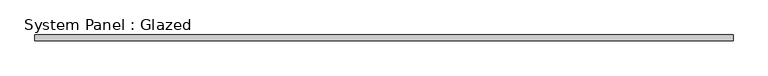
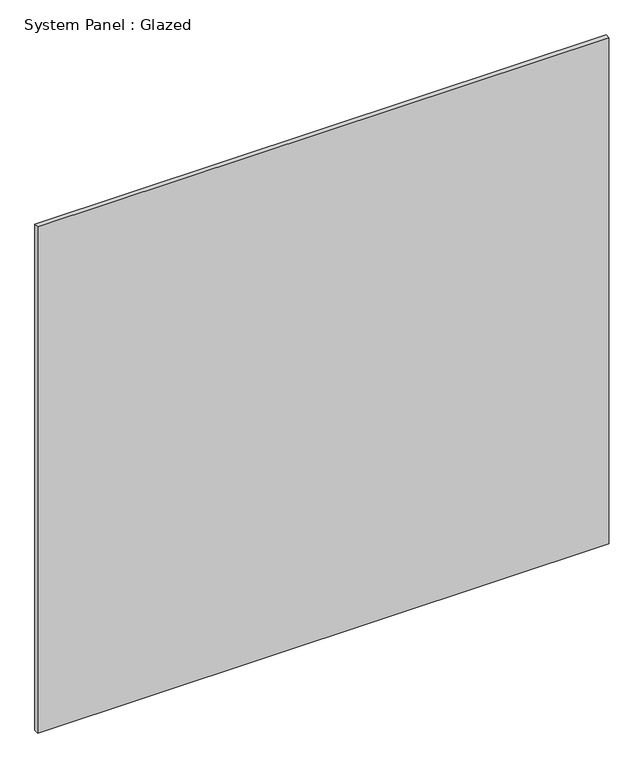
"""IFC4 building model written with IfcOpenShell, lengths in millimetres: plate geometry, System Panel : Glazed."""

from ifc_helpers import new_model, si_unit, origin, origin_with_axes, place, context, project, spatial, polyline, outline, extrude, source, transform, mapped, element, save


def system_panel_glazed_34d630f4(model_context):
    return source(origin(), model_context, "Body", "SweptSolid", [
        extrude(outline(polyline([(1558.2120883, 19.05), (-1558.2120883, 19.05), (-1558.2120883, 44.45), (1558.2120883, 44.45), (1558.2120883, 19.05)])), origin_with_axes(), (0.0, 0.0, 1.0), 2921.0),
    ])


if __name__ == "__main__":
    model = new_model("IFC4")
    model_context = context("Model", 3, world=origin())
    ifc_project = project(units=[si_unit("LENGTHUNIT", "METRE", prefix="MILLI")], contexts=[model_context])
    site = spatial("IfcSite", under=ifc_project)
    building = spatial("IfcBuilding", under=site)
    placement = place(None, origin())
    system_panel_glazed_shape = system_panel_glazed_34d630f4(model_context)
    element("IfcPlate", 1, ObjectType="System Panel : Glazed", at=placement, inside=building, context=model_context, shape_type="MappedRepresentation", body=[
        mapped(system_panel_glazed_shape, transform((0.0, 0.0, 0.0), x_axis=(1.0, 0.0, 0.0), y_axis=(0.0, 1.0, 0.0), z_axis=(0.0, 0.0, 1.0))),
    ])
    save(model, "model.ifc")

# Revit data of these elements
# Type "System Panel : Glazed"
#   Construction Type Id = "GSP4R"
#   Analytic Construction = "1/8 in Pilkington single glazing"
#   Visual Light Transmittance = 0.9
#   Solar Heat Gain Coefficient = 0.86
#   Heat Transfer Coefficient (U) = 1.18115 BTU/(h·ft²·°F)
#   Define Thermal Properties by = 1
# Element 1 (IfcPlate, "System Panel : Glazed")
#   Materials on its faces: "Glass"
# Materials
#   "Glass": class "Glass", colour RGB 0 128 192, transparency 0.75, Description = "Soda Lime Glass", Cost = 0
